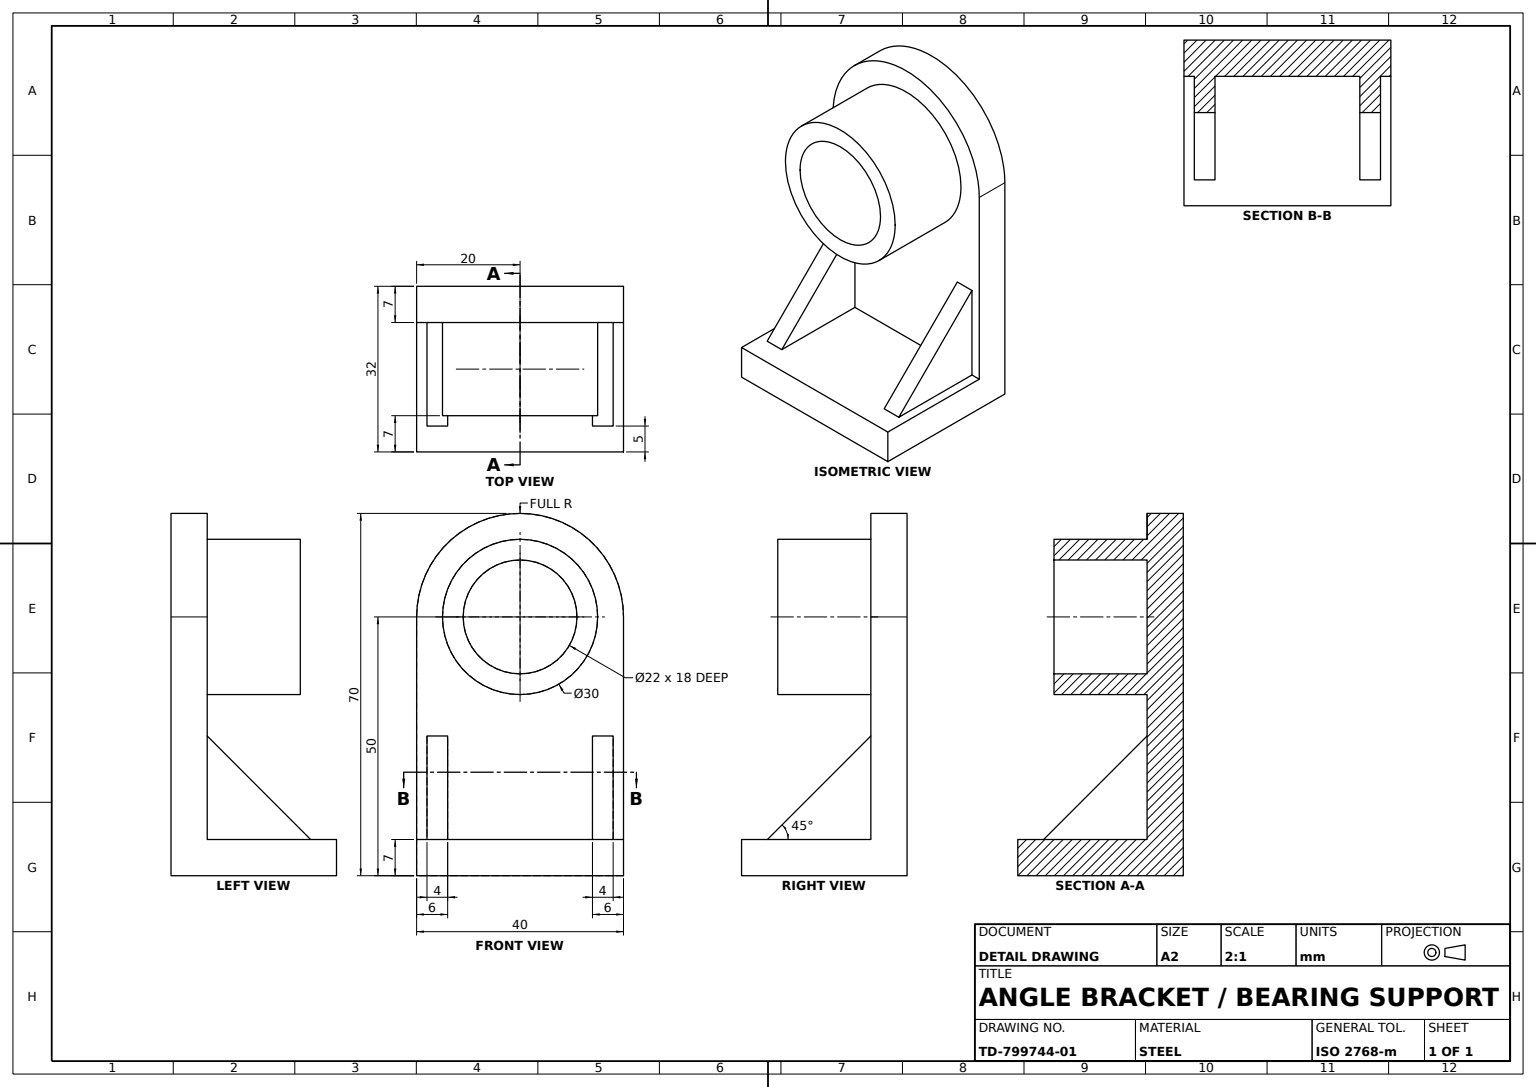
SolidWorks part; units mm, degrees
material "Plain Carbon Steel"
ref_plane "Front Plane" through (0, 0, 0) normal (0, 0, 1) x (1, 0, 0)
ref_plane "Top Plane" through (0, 0, 0) normal (0, 1, 0) x (1, 0, 0)
ref_plane "Right Plane" through (0, 0, 0) normal (1, 0, 0) x (0, 0, -1)
sketch "Base Angle Profile Sketch" plane through (0, 0, 0) normal (1, 0, 0) x (0, 0, -1)
  line L0 (-817.4085, 0) -> (40053.0162, 0) construction
  line L1 (0, -817.4085) -> (0, 40053.0162) construction
  line L2 (0, 0) -> (32, 0)
  line L3 (32, 0) -> (32, 50)
  line L4 (32, 50) -> (25, 50)
  line L5 (25, 50) -> (25, 7)
  line L6 (25, 7) -> (0, 7)
  line L7 (0, 7) -> (0, 0)
  dimension "D1" = 32
  dimension "D2" = 7
  dimension "D3" = 7
  dimension "D4" = 50
extrude "Base Angle" add sketch "Base Angle Profile Sketch" along normal mid plane 40
sketch "Upright Plate Sketch" plane through (0, 0, -25) normal (0, 0, 1) x (1, 0, 0)
  line L4 (-20, 50) -> (-20, 7)
  line L5 (-20, 7) -> (20, 7)
  line L6 (20, 7) -> (20, 50)
  line L7 (20, 50) -> (-20, 50)
  line L8 (-20, 50) -> (-20, 7)
  line L9 (-20, 7) -> (20, 7)
  line L10 (20, 7) -> (20, 50)
  arc A0 (-20, 50) -> (20, 50) centre (0, 50) cw
  dimension "D1" = 20
  dimension "D2" = 0
extrude "Upright Plate" add sketch "Upright Plate Sketch" against normal blind 7 contours A0 L5
sketch "Bearing Hub Sketch" plane through (0, 0, -25) normal (0, 0, 1) x (1, 0, 0)
  circle A0 centre (0, 50) radius 15
  circle A1 centre (0, 50) radius 11
  dimension "D1" = 22
  dimension "D2" = 30
extrude "Bearing Hub Ø30 Bore Ø22" add sketch "Bearing Hub Sketch" along normal blind 18
sketch "Gusset Rib Sketch" plane through (20, 0, 0) normal (1, 0, 0) x (0, 0, -1)
  line L0 (5, 7) -> (25, 27)
  line L1 (25, 7) -> (0, 7) construction
  line L2 (25, 50) -> (25, 7) construction
  line L3 (25, 27) -> (25, 7)
  line L4 (25, 7) -> (5, 7)
  dimension "D1" = 20
  dimension "D2" = 20
extrude "Gusset Rib" add sketch "Gusset Rib Sketch" along normal blind 4 from offset 6 offset against normal yes
mirror "Gusset Rib Mirror" about plane through (0, 0, 0) normal (1, 0, 0) of "Gusset Rib"
